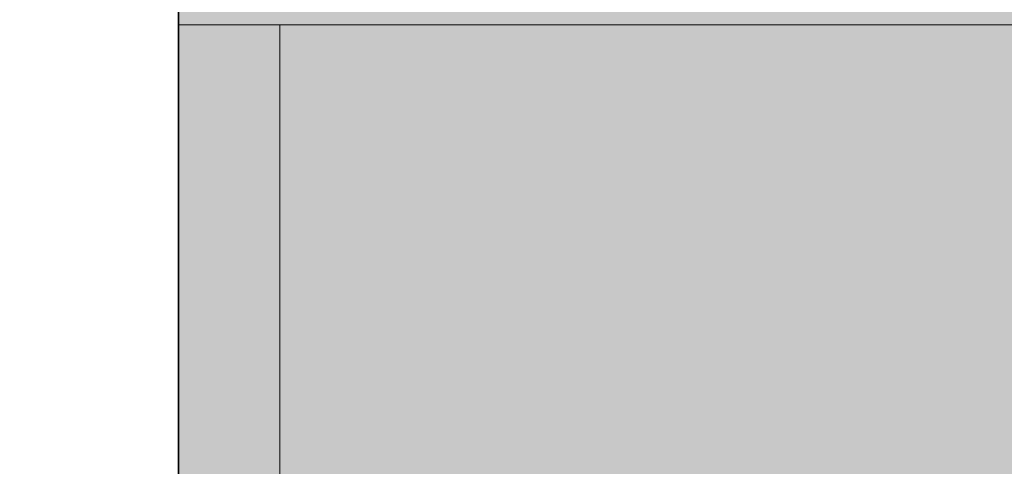
# Model space of a CAD drawing. Units: inches. Extents: x 1704 to 6393, y -157 to 1172.
# Tile 53 of 122: x 1892 to 1931, y 870 to 887. Entities that reach past the tile are written whole.
import ezdxf

# ---------------------------------------------------------------- set-up
doc = ezdxf.new("R2010")
doc.units = ezdxf.units.IN
doc.header["$MEASUREMENT"] = 0
for name, color, linetype, lineweight in [('A-ANNO-DIMS', 7, 'Continuous', 13), ('C-PROP', 7, 'Continuous', 35), ('L-HRDS', 8, 'Continuous', 18)]:
    doc.layers.add(name, color=color, linetype=linetype, lineweight=lineweight)
doc.layers.add('L-HRDS-PATT', color=9, linetype='Continuous', lineweight=13, true_color=0xc5c1ba)
doc.layers.add('L-WATR-PATT', color=143, linetype='Continuous', lineweight=13, true_color=0x7ab0df)
doc.styles.get("Standard").update_dxf_attribs({"font": 'arial.ttf'})
doc.dimstyles.get("Standard").update_dxf_attribs({"dimtxt": 6, "dimasz": 2, "dimexe": 0.18, "dimexo": 0.0625, "dimgap": 0.09, "dimtad": 0, "dimtih": 1, "dimtoh": 1, "dimdec": 1, "dimzin": 0, "dimdsep": 46, "dimlunit": 3, "dimtxsty": 'Standard', "dimblk": 'ARCHTICK', "dimcen": 0.09, "dimadec": 0, "dimazin": 0, "dimtfac": 1, "dimtdec": 1, "dimtofl": 0, "dimtmove": 0, "dimatfit": 3, "dimfxl": 1, "dimtolj": 1, "dimtzin": 0, "dimarcsym": 0})

# ---------------------------------------------------------------- blocks, each defined once
blk = doc.blocks.new('_ArchTick')
at = {"color": 0, "linetype": 'ByBlock', "const_width": 0.15}
blk.add_lwpolyline([(-0.5, -0.5), (0.5, 0.5)], dxfattribs=at)
blk = doc.blocks.new('*D93')
at = {"layer": 'A-ANNO-DIMS', "color": 0, "lineweight": -2, "transparency": 16777216}
for p, q in [((2605.286, 895.213), (1829.698, 895.213)), ((1829.878, 895.213), (1829.878, 495.866)), ((1829.878, 90.213), (1829.878, 489.56)), ((2605.286, 90.213), (1829.698, 90.213))]:
    blk.add_line(p, q, dxfattribs=at)
at = {"layer": 'Defpoints', "color": 0, "lineweight": -3, "transparency": 16777216}
for p in [(2605.349, 895.213), (1829.878, 90.213), (2605.349, 90.213)]:
    blk.add_point(p, dxfattribs=at)
at = {"layer": 'A-ANNO-DIMS', "color": 0, "lineweight": -2, "transparency": 16777216, "xscale": 2, "yscale": 2, "zscale": 2}
for p, rotation in [((1829.878, 895.213), 90), ((1829.878, 90.213), 270)]:
    blk.add_blockref('_ArchTick', p, dxfattribs=dict(at, rotation=rotation))
at = {"layer": 'A-ANNO-DIMS', "color": 0, "transparency": 16777216, "insert": (1829.878, 492.713), "char_height": 6, "attachment_point": 5}
blk.add_mtext('\\A1;805', dxfattribs=at)

msp = doc.modelspace()

# ---------------------------------------------------------------- hatches: boundary and pattern name
at = {"layer": 'L-HRDS-PATT', "transparency": 33554643}
h = msp.add_hatch(color=256, dxfattribs=at)
h.dxf.hatch_style = 1
h.paths.add_polyline_path([(2073.349, 719.213), (2021.151, 719.213), (2021.151, 711.213), (2073.349, 711.213)])
h.paths.add_polyline_path([(1977.349, 719.213), (1969.349, 719.213), (1898.349, 719.213), (1898.349, 711.213), (1977.349, 711.213)])
h.paths.add_polyline_path([(1977.349, 895.213), (1898.349, 895.213), (1898.349, 887.213), (1969.349, 887.213), (1977.349, 887.213)])
at = {"layer": 'L-HRDS-PATT'}
h = msp.add_hatch(color=256, dxfattribs=at)
h.dxf.hatch_style = 1
h.paths.add_polyline_path([(1902.349, 887.213), (1898.349, 887.213), (1898.349, 719.213), (1902.349, 719.213)])
at = {"layer": 'L-WATR-PATT'}
h = msp.add_hatch(color=256, dxfattribs=at)
h.dxf.hatch_style = 1
h.paths.add_polyline_path([(1969.349, 887.213), (1902.349, 887.213), (1902.349, 719.213), (1969.349, 719.213)])

# ---------------------------------------------------------------- linework, layer by layer
at = {"layer": 'C-PROP'}
msp.add_line((1898.349, -3.787), (1898.349, 1033.213), dxfattribs=at)
at = {"layer": 'L-HRDS'}
for p, q in [((1969.349, 887.213), (1898.349, 887.213)), ((1902.349, 887.213), (1902.349, 719.213))]:
    msp.add_line(p, q, dxfattribs=at)

# ---------------------------------------------------------------- dimensions: what is measured, and where the dimension line sits
at = {"layer": 'A-ANNO-DIMS'}
dim = msp.add_linear_dim(base=(1829.878, 90.213), p1=(2605.349, 895.213), p2=(2605.349, 90.213), angle=90, dimstyle='Standard', override={"dimdec": 0, "dimlfac": 1, "dimrnd": 0, "dimzin": 0, "dimdsep": 46, "dimlunit": 2}, dxfattribs=at)
dim.commit()
dim.dimension.update_dxf_attribs({"geometry": '*D93', "text_midpoint": (1829.878, 492.713)})

doc.saveas('drawing.dxf')
